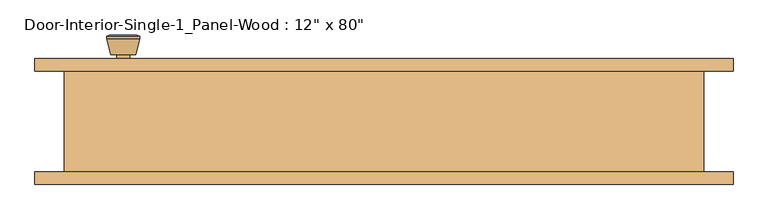
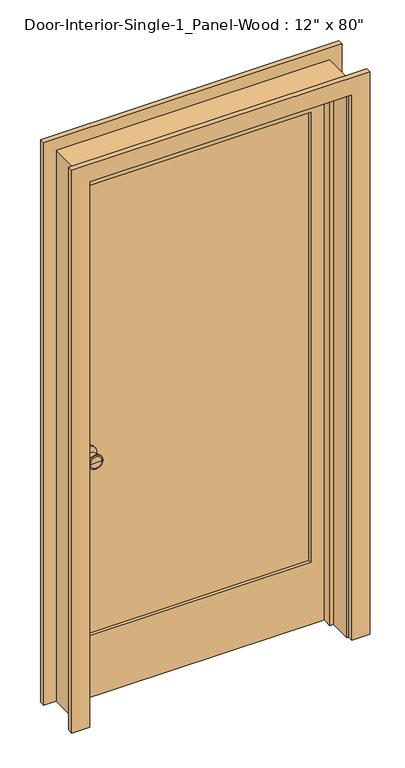
"""IFC4 building model written with IfcOpenShell, lengths in millimetres: door geometry."""

from ifc_helpers import new_model, si_unit, point, frame, frame_2d, origin, place, context, project, spatial, polyline, circle_curve, trimmed, segment, composite_curve, outline, extrude, faceted_brep, source, transform, mapped, element, save
from ifc_brep_helpers import plane_surface, cylinder_surface, revolved_surface, advanced_brep


def door_b28d7136(model_context):
    return source(origin(), model_context, "Body", "SolidModel", [
        advanced_brep(
        [(-393.7, 32.1, 914.4), (-383.7, 32.1, 914.4), (-403.7, 32.1, 914.4), (-373.2241324, -16.9, 914.4), (-393.7, -16.9, 914.4), (-414.1758676, -16.9, 914.4), (-368.7, -15.0721319, 914.4), (-418.7, -15.0721319, 914.4), (-368.7, -11.6084537, 914.4), (-418.7, -11.6084537, 914.4), (-375.063764, 13.1, 914.4), (-412.336236, 13.1, 914.4), (-383.7, 13.1, 914.4), (-403.7, 13.1, 914.4)],
        [
            (0, 1),
            (1, 2, circle_curve(frame((-393.7, 32.1, 914.4), z_axis=(0.0, 1.0, 0.0), x_axis=(-1.0, 0.0, 0.0)), 10.0)),
            (2, 0),
            (2, 1, circle_curve(frame((-393.7, 32.1, 914.4), z_axis=(0.0, 1.0, 0.0), x_axis=(-1.0, 0.0, 0.0)), 10.0)),
            (3, 4),
            (4, 5),
            (5, 3, circle_curve(frame((-393.7, -16.9, 914.4), z_axis=(0.0, -1.0, 0.0), x_axis=(-1.0, 0.0, 0.0)), 20.4758676)),
            (3, 5, circle_curve(frame((-393.7, -16.9, 914.4), z_axis=(0.0, -1.0, 0.0), x_axis=(-1.0, 0.0, 0.0)), 20.4758676)),
            (6, 3),
            (5, 7),
            (7, 6, circle_curve(frame((-393.7, -15.0721319, 914.4), z_axis=(0.0, -1.0, 0.0), x_axis=(-1.0, 0.0, 0.0)), 25.0)),
            (6, 7, circle_curve(frame((-393.7, -15.0721319, 914.4), z_axis=(0.0, -1.0, 0.0), x_axis=(-1.0, 0.0, 0.0)), 25.0)),
            (8, 6),
            (7, 9),
            (9, 8, circle_curve(frame((-393.7, -11.6084537, 914.4), z_axis=(0.0, -1.0, 0.0), x_axis=(-1.0, 0.0, 0.0)), 25.0)),
            (8, 9, circle_curve(frame((-393.7, -11.6084537, 914.4), z_axis=(0.0, -1.0, 0.0), x_axis=(-1.0, 0.0, 0.0)), 25.0)),
            (10, 8),
            (9, 11),
            (11, 10, circle_curve(frame((-393.7, 13.1, 914.4), z_axis=(0.0, -1.0, 0.0), x_axis=(-1.0, 0.0, 0.0)), 18.636236)),
            (10, 11, circle_curve(frame((-393.7, 13.1, 914.4), z_axis=(0.0, -1.0, 0.0), x_axis=(-1.0, 0.0, 0.0)), 18.636236)),
            (12, 10),
            (11, 13),
            (13, 12, circle_curve(frame((-393.7, 13.1, 914.4), z_axis=(0.0, -1.0, 0.0), x_axis=(-1.0, 0.0, 0.0)), 10.0)),
            (12, 13, circle_curve(frame((-393.7, 13.1, 914.4), z_axis=(0.0, -1.0, 0.0), x_axis=(-1.0, 0.0, 0.0)), 10.0)),
            (1, 12),
            (13, 2),
        ],
        [
            plane_surface(frame((-393.7, 32.1, 914.4), z_axis=(0.0, 1.0, 0.0), x_axis=(-1.0, 0.0, 0.0))),
            plane_surface(frame((-393.7, -16.9, 914.4), z_axis=(0.0, -1.0, 0.0), x_axis=(-1.0, 0.0, 0.0))),
            revolved_surface(polyline([(-414.1758676, -16.9, 914.4), (-418.7, -15.0721319, 914.4)]), (-393.7, 32.1, 914.4), (0.0, 1.0, 0.0)),
            cylinder_surface(frame((-393.7, 32.1, 914.4), z_axis=(0.0, 1.0, 0.0), x_axis=(-1.0, 0.0, 0.0)), 25.0),
            revolved_surface(polyline([(-418.7, -11.6084537, 914.4), (-412.336236, 13.1, 914.4)]), (-393.7, 32.1, 914.4), (0.0, 1.0, 0.0)),
            plane_surface(frame((-393.7, 13.1, 914.4), z_axis=(0.0, 1.0, 0.0), x_axis=(-1.0, 0.0, 0.0))),
            cylinder_surface(frame((-393.7, 32.1, 914.4), z_axis=(0.0, 1.0, 0.0), x_axis=(-1.0, 0.0, 0.0)), 10.0),
        ],
        [
            (0, [[1, 2, 3]]),
            (0, [[-3, 4, -1]]),
            (1, [[5, 6, 7]]),
            (1, [[-6, -5, 8]]),
            (2, [[9, -7, 10, 11]]),
            (2, [[-10, -8, -9, 12]]),
            (3, [[13, -11, 14, 15]]),
            (3, [[-14, -12, -13, 16]]),
            (4, [[17, -15, 18, 19]]),
            (4, [[-18, -16, -17, 20]]),
            (5, [[21, -19, 22, 23]]),
            (5, [[-22, -20, -21, 24]]),
            (6, [[25, -23, 26, -2]]),
            (6, [[-26, -24, -25, -4]]),
        ],
    ),
        extrude(outline(composite_curve([segment(trimmed(circle_curve(frame_2d((914.4, -393.7)), 30.0), [point((914.4, -423.7))], [point((914.4, -363.7))], False, "CARTESIAN"), True, "CONTINUOUS"), segment(trimmed(circle_curve(frame_2d((914.4, -393.7)), 30.0), [point((914.4, -363.7))], [point((914.4, -423.7))], False, "CARTESIAN"), True, "CONTINUOUS")], self_intersect=False)), frame((0.0, 32.1, 0.0), z_axis=(0.0, 1.0, 0.0), x_axis=(0.0, 0.0, 1.0)), (0.0, 0.0, 1.0), 6.0),
        advanced_brep(
        [(-393.7, 79.025, 914.4), (-403.7, 79.025, 914.4), (-383.7, 79.025, 914.4), (-373.2241324, 128.025, 914.4), (-414.1758676, 128.025, 914.4), (-393.7, 128.025, 914.4), (-368.7, 126.1971319, 914.4), (-418.7, 126.1971319, 914.4), (-368.7, 122.7334537, 914.4), (-418.7, 122.7334537, 914.4), (-375.063764, 98.025, 914.4), (-412.336236, 98.025, 914.4), (-383.7, 98.025, 914.4), (-403.7, 98.025, 914.4)],
        [
            (0, 1),
            (1, 2, circle_curve(frame((-393.7, 79.025, 914.4), z_axis=(0.0, -1.0, 0.0), x_axis=(-1.0, 0.0, 0.0)), 10.0)),
            (2, 0),
            (2, 1, circle_curve(frame((-393.7, 79.025, 914.4), z_axis=(0.0, -1.0, 0.0), x_axis=(-1.0, 0.0, 0.0)), 10.0)),
            (3, 4, circle_curve(frame((-393.7, 128.025, 914.4), z_axis=(0.0, 1.0, 0.0), x_axis=(-1.0, 0.0, 0.0)), 20.4758676)),
            (4, 5),
            (5, 3),
            (4, 3, circle_curve(frame((-393.7, 128.025, 914.4), z_axis=(0.0, 1.0, 0.0), x_axis=(-1.0, 0.0, 0.0)), 20.4758676)),
            (6, 7, circle_curve(frame((-393.7, 126.1971319, 914.4), z_axis=(0.0, 1.0, 0.0), x_axis=(-1.0, 0.0, 0.0)), 25.0)),
            (7, 4),
            (3, 6),
            (7, 6, circle_curve(frame((-393.7, 126.1971319, 914.4), z_axis=(0.0, 1.0, 0.0), x_axis=(-1.0, 0.0, 0.0)), 25.0)),
            (8, 9, circle_curve(frame((-393.7, 122.7334537, 914.4), z_axis=(0.0, 1.0, 0.0), x_axis=(-1.0, 0.0, 0.0)), 25.0)),
            (9, 7),
            (6, 8),
            (9, 8, circle_curve(frame((-393.7, 122.7334537, 914.4), z_axis=(0.0, 1.0, 0.0), x_axis=(-1.0, 0.0, 0.0)), 25.0)),
            (10, 11, circle_curve(frame((-393.7, 98.025, 914.4), z_axis=(0.0, 1.0, 0.0), x_axis=(-1.0, 0.0, 0.0)), 18.636236)),
            (11, 9),
            (8, 10),
            (11, 10, circle_curve(frame((-393.7, 98.025, 914.4), z_axis=(0.0, 1.0, 0.0), x_axis=(-1.0, 0.0, 0.0)), 18.636236)),
            (12, 13, circle_curve(frame((-393.7, 98.025, 914.4), z_axis=(0.0, 1.0, 0.0), x_axis=(-1.0, 0.0, 0.0)), 10.0)),
            (13, 11),
            (10, 12),
            (13, 12, circle_curve(frame((-393.7, 98.025, 914.4), z_axis=(0.0, 1.0, 0.0), x_axis=(-1.0, 0.0, 0.0)), 10.0)),
            (1, 13),
            (12, 2),
        ],
        [
            plane_surface(frame((-393.7, 79.025, 914.4), z_axis=(0.0, -1.0, 0.0), x_axis=(-1.0, 0.0, 0.0))),
            plane_surface(frame((-393.7, 128.025, 914.4), z_axis=(0.0, 1.0, 0.0), x_axis=(-1.0, 0.0, 0.0))),
            revolved_surface(polyline([(-414.1758676, 128.025, 914.4), (-418.7, 126.1971319, 914.4)]), (-393.7, 79.025, 914.4), (0.0, -1.0, 0.0)),
            cylinder_surface(frame((-393.7, 79.025, 914.4), z_axis=(0.0, -1.0, 0.0), x_axis=(-1.0, 0.0, 0.0)), 25.0),
            revolved_surface(polyline([(-418.7, 122.7334537, 914.4), (-412.336236, 98.025, 914.4)]), (-393.7, 79.025, 914.4), (0.0, -1.0, 0.0)),
            plane_surface(frame((-393.7, 98.025, 914.4), z_axis=(0.0, -1.0, 0.0), x_axis=(-1.0, 0.0, 0.0))),
            cylinder_surface(frame((-393.7, 79.025, 914.4), z_axis=(0.0, -1.0, 0.0), x_axis=(-1.0, 0.0, 0.0)), 10.0),
        ],
        [
            (0, [[1, 2, 3]]),
            (0, [[-3, 4, -1]]),
            (1, [[5, 6, 7]]),
            (1, [[8, -7, -6]]),
            (2, [[9, 10, -5, 11]]),
            (2, [[12, -11, -8, -10]]),
            (3, [[13, 14, -9, 15]]),
            (3, [[16, -15, -12, -14]]),
            (4, [[17, 18, -13, 19]]),
            (4, [[20, -19, -16, -18]]),
            (5, [[21, 22, -17, 23]]),
            (5, [[24, -23, -20, -22]]),
            (6, [[-2, 25, -21, 26]]),
            (6, [[-4, -26, -24, -25]]),
        ],
    ),
        extrude(outline(composite_curve([segment(trimmed(circle_curve(frame_2d((914.4, -393.7)), 30.0), [point((914.4, -423.7))], [point((914.4, -363.7))], False, "CARTESIAN"), True, "CONTINUOUS"), segment(trimmed(circle_curve(frame_2d((914.4, -393.7)), 30.0), [point((914.4, -363.7))], [point((914.4, -423.7))], False, "CARTESIAN"), True, "CONTINUOUS")], self_intersect=False)), frame((0.0, 73.025, 0.0), z_axis=(0.0, 1.0, 0.0), x_axis=(0.0, 0.0, 1.0)), (0.0, 0.0, 1.0), 6.0),
        extrude(outline(polyline([(396.875, 49.7416667), (-396.875, 49.7416667), (-396.875, 61.3833333), (396.875, 61.3833333), (396.875, 49.7416667)])), frame((0.0, 0.0, 231.775), z_axis=(0.0, 0.0, 1.0), x_axis=(1.0, 0.0, 0.0)), (0.0, 0.0, 1.0), 1681.1625),
        extrude(outline(polyline([(2032.0, -457.2), (0.0, -457.2), (0.0, 457.2), (2032.0, 457.2), (2032.0, -457.2)]), holes=[polyline([(1912.9375, -396.875), (1912.9375, 396.875), (231.775, 396.875), (231.775, -396.875), (1912.9375, -396.875)])]), frame((0.0, 38.1, 0.0), z_axis=(0.0, 1.0, 0.0), x_axis=(0.0, 0.0, 1.0)), (0.0, 0.0, 1.0), 34.925),
        faceted_brep([(482.6, 73.025, 0.0), (482.6, -79.375, 0.0), (457.2, -79.375, 0.0), (457.2, 3.175, 0.0), (444.5, 3.175, 0.0), (444.5, 38.1, 0.0), (457.2, 38.1, 0.0), (457.2, 73.025, 0.0), (482.6, 73.025, 2057.4), (482.6, -79.375, 2057.4), (-482.6, -79.375, 2057.4), (-482.6, -79.375, 0.0), (-457.2, -79.375, 0.0), (-457.2, -79.375, 2032.0), (457.2, -79.375, 2032.0), (457.2, 3.175, 2032.0), (-457.2, 3.175, 2032.0), (-457.2, 3.175, 0.0), (-444.5, 3.175, 0.0), (-444.5, 3.175, 2019.3), (444.5, 3.175, 2019.3), (444.5, 38.1, 2019.3), (-444.5, 38.1, 2019.3), (-444.5, 38.1, 0.0), (-457.2, 38.1, 0.0), (-457.2, 38.1, 2032.0), (457.2, 38.1, 2032.0), (457.2, 73.025, 2032.0), (-457.2, 73.025, 2032.0), (-457.2, 73.025, 0.0), (-482.6, 73.025, 0.0), (-482.6, 73.025, 2057.4)], [[[0, 1, 2, 3, 4, 5, 6, 7]], [[1, 0, 8, 9]], [[2, 1, 9, 10, 11, 12, 13, 14]], [[3, 2, 14, 15]], [[4, 3, 15, 16, 17, 18, 19, 20]], [[5, 4, 20, 21]], [[6, 5, 21, 22, 23, 24, 25, 26]], [[7, 6, 26, 27]], [[0, 7, 27, 28, 29, 30, 31, 8]], [[9, 8, 31, 10]], [[15, 14, 13, 16]], [[21, 20, 19, 22]], [[27, 26, 25, 28]], [[30, 29, 24, 23, 18, 17, 12, 11]], [[10, 31, 30, 11]], [[16, 13, 12, 17]], [[22, 19, 18, 23]], [[28, 25, 24, 29]]]),
        extrude(outline(polyline([(0.0, 463.55), (0.0, 527.05), (2101.85, 527.05), (2101.85, -527.05), (0.0, -527.05), (0.0, -463.55), (2038.35, -463.55), (2038.35, 463.55), (0.0, 463.55)])), frame((0.0, -98.425, 0.0), z_axis=(0.0, 1.0, 0.0), x_axis=(0.0, 0.0, 1.0)), (0.0, 0.0, 1.0), 19.05),
        extrude(outline(polyline([(0.0, 463.55), (0.0, 527.05), (2101.85, 527.05), (2101.85, -527.05), (0.0, -527.05), (0.0, -463.55), (2038.35, -463.55), (2038.35, 463.55), (0.0, 463.55)])), frame((0.0, 73.025, 0.0), z_axis=(0.0, 1.0, 0.0), x_axis=(0.0, 0.0, 1.0)), (0.0, 0.0, 1.0), 19.05),
    ])


if __name__ == "__main__":
    model = new_model("IFC4")
    model_context = context("Model", 3, world=origin())
    ifc_project = project(units=[si_unit("LENGTHUNIT", "METRE", prefix="MILLI")], contexts=[model_context])
    site = spatial("IfcSite", under=ifc_project)
    building = spatial("IfcBuilding", under=site)
    placement = place(None, origin())
    door_shape = door_b28d7136(model_context)
    element("IfcDoor", 1, ObjectType="Door-Interior-Single-1_Panel-Wood : 12\" x 80\"", at=placement, inside=building, context=model_context, shape_type="MappedRepresentation", body=[
        mapped(door_shape, transform((0.0, 0.0, 0.0), x_axis=(1.0, 0.0, 0.0), y_axis=(0.0, 1.0, 0.0), z_axis=(0.0, 0.0, 1.0))),
    ])
    save(model, "model.ifc")

# Revit data of these elements
# Type "Door-Interior-Single-1_Panel-Wood : 12\" x 80\""
#   Type Mark = "9"
#   Assembly Code = "C1020300"
#   Analytic Construction = "Wooden"
#   Top Rail = 0' - 4 11/16"
#   Thickness = 0' - 1 3/8"
#   Thermal Resistance (R) = 2.5876 (h·ft²·°F)/BTU
#   Swing Angle [instance default] = 90.00°
#   Stiles = 0' - 2 3/8"
#   Rough Width = 3' - 2"
#   Rough Height = 6' - 9"
#   Height = 6' - 8"
#   Width = 3' - 0"
#   Heat Transfer Coefficient (U) = 0.3865 BTU/(h·ft²·°F)
#   Bottom Rail = 0' - 9 1/8"
#   Trim Material = Cherry
#   Panel Material = Cherry
#   Frame Material = Cherry
#   Door Handle Material = Aluminum
#   Visual Light Transmittance = 0
#   Solar Heat Gain Coefficient = 0
#   Wall Closure = (empty or 0)
#   Function = (empty or 0)
# Element 1 (IfcDoor, "Door-Interior-Single-1_Panel-Wood : 12\" x 80\"")
#   Materials on its faces: "Cherry", "Aluminum"
# Materials
#   "Cherry": class "Wood", colour RGB 226 177 128, transparency 0, Description = "Prunus Serotina", Cost = 0
#   "Aluminum": class "Metal", colour RGB 247 247 247, transparency 0, Description = "Aluminum 6061", Cost = 0
